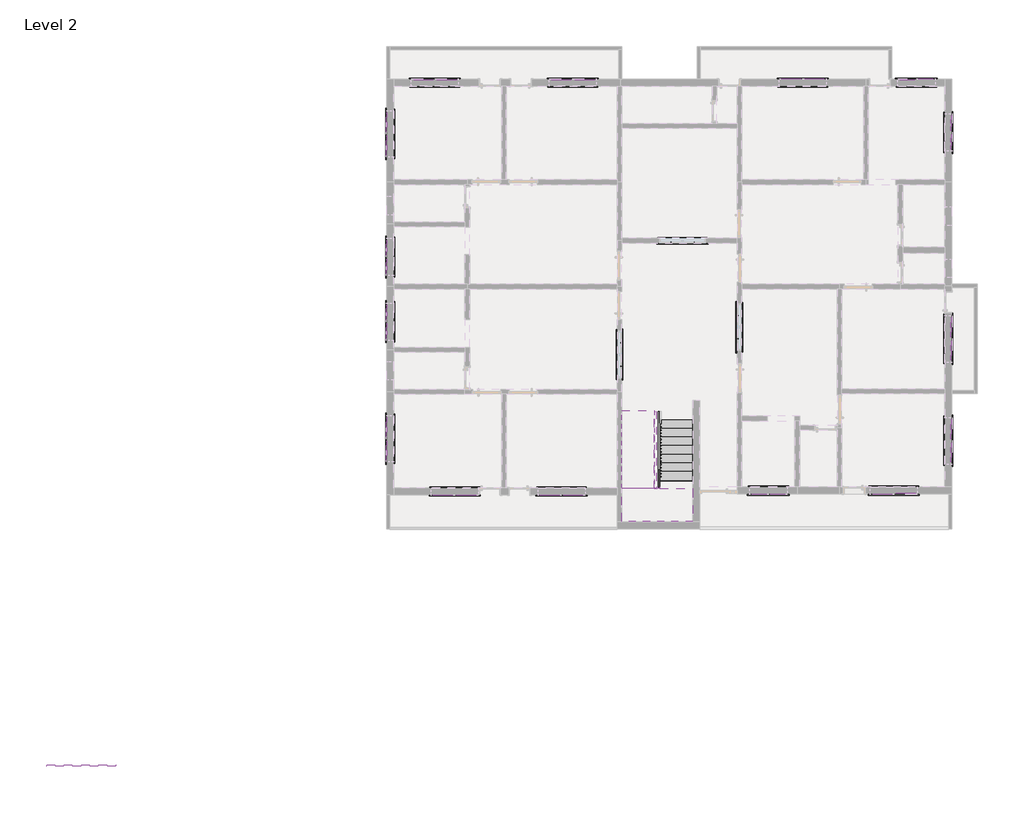
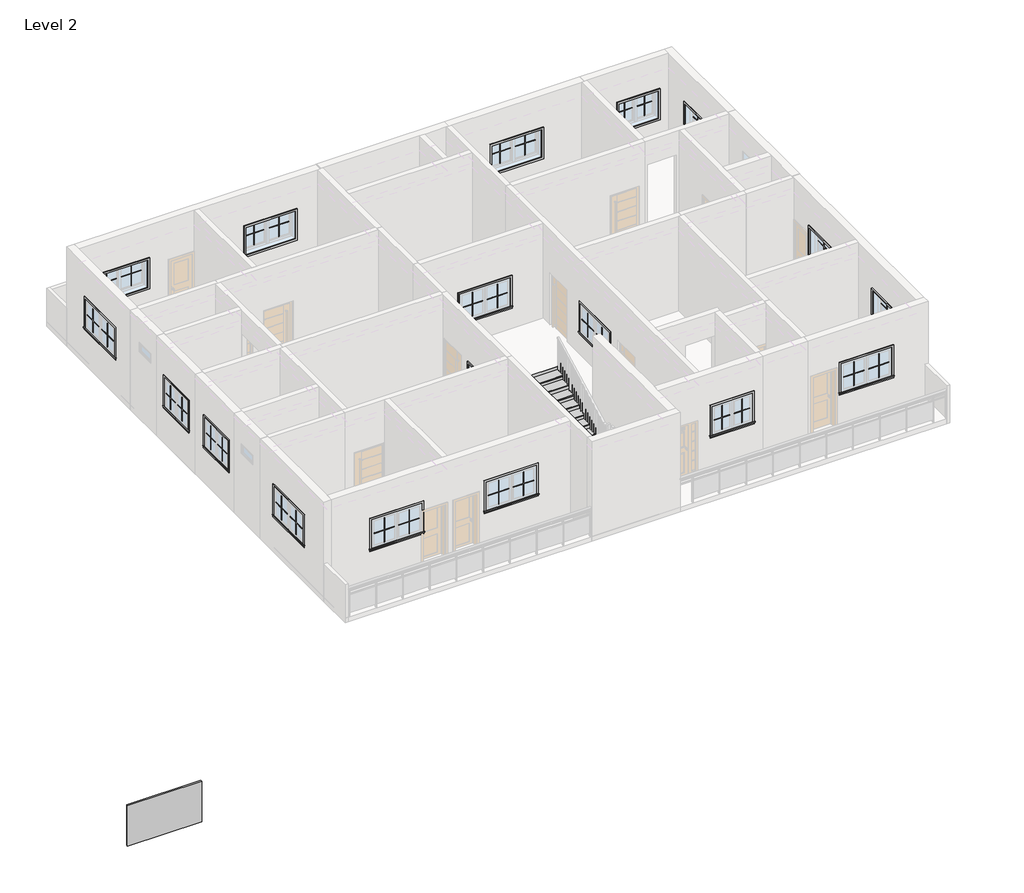
# One storey, part 5 of 5: 73 proxies, 3 members, 2 stair flights, 1 slab.
"""IFC4 building model written with IfcOpenShell, lengths in millimetres."""

from ifc_helpers import new_model, si_unit, frame, origin, place, context, project, spatial, polyline, outline, extrude, transform, mapped, element, save
from components import flag_flag_4961f895, m_muntin_pattern_2x2_m_muntin_pattern_2x2_9352d081, m_muntin_pattern_2x2_m_muntin_pattern_2x2_5c2cbe28, m_muntin_pattern_2x2_m_muntin_pattern_2x2_2357e71d, m_muntin_pattern_2x2_m_muntin_pattern_2x2_302d8f29, m_trim_window_exterior_flat_with_sill_e3533f3c, m_trim_window_exterior_flat_with_sill_6ae8fed8, m_trim_window_interior_flat_picture_frame_7d8195fd, m_trim_window_interior_flat_picture_frame_fffd0b6f, non_monolithic_landing_175d1c90, stair_flight_4edc9e4a, stair_flight_4fea8275

model = new_model("IFC4")

# Units and contexts
model_context = context("Model", 3, world=origin())
ifc_project = project(units=[si_unit("LENGTHUNIT", "METRE", prefix="MILLI")], contexts=[model_context])

# Site, building, storey
site = spatial("IfcSite", under=ifc_project)
building = spatial("IfcBuilding", under=site)
storey = spatial("IfcBuildingStorey", under=building, Name="Level 2", Elevation=3200.4)

# Proxies
placement = place(None, origin())
flag_flag_shape = flag_flag_4961f895(model_context)
element("IfcBuildingElementProxy", 1, Name="FLAG : FLAG", ObjectType="FLAG : FLAG", at=placement, inside=storey, context=model_context, shape_type="MappedRepresentation", body=[
    mapped(flag_flag_shape, transform((0.0, 0.0, 0.0), x_axis=(1.0, 0.0, 0.0), y_axis=(0.0, 1.0, 0.0), z_axis=(0.0, 0.0, 1.0))),
])
m_muntin_pattern_2x2_m_muntin_pattern_2x2_shape = m_muntin_pattern_2x2_m_muntin_pattern_2x2_9352d081(model_context)
element("IfcBuildingElementProxy", 2, Name="M_Muntin Pattern_2x2 : M_Muntin Pattern_2x2", ObjectType="M_Muntin Pattern_2x2 : M_Muntin Pattern_2x2", at=placement, inside=storey, context=model_context, shape_type="MappedRepresentation", body=[
    mapped(m_muntin_pattern_2x2_m_muntin_pattern_2x2_shape, transform((-23821.9972893, 23321.4672903, 4489.4070312), x_axis=(1.0, 0.0, 0.0), y_axis=(0.0, 1.0, 0.0), z_axis=(0.0, 0.0, 1.0))),
])
element("IfcBuildingElementProxy", 3, Name="M_Muntin Pattern_2x2 : M_Muntin Pattern_2x2", ObjectType="M_Muntin Pattern_2x2 : M_Muntin Pattern_2x2", at=placement, inside=storey, context=model_context, shape_type="MappedRepresentation", body=[
    mapped(m_muntin_pattern_2x2_m_muntin_pattern_2x2_shape, transform((-24995.1597893, 21173.5797903, 4489.4070312), x_axis=(0.0, 1.0, 0.0), y_axis=(-1.0, 0.0, 0.0), z_axis=(0.0, 0.0, 1.0))),
])
element("IfcBuildingElementProxy", 4, Name="M_Muntin Pattern_2x2 : M_Muntin Pattern_2x2", ObjectType="M_Muntin Pattern_2x2 : M_Muntin Pattern_2x2", at=placement, inside=storey, context=model_context, shape_type="MappedRepresentation", body=[
    mapped(m_muntin_pattern_2x2_m_muntin_pattern_2x2_shape, transform((-24995.1597893, 11242.1797903, 4489.4070312), x_axis=(0.0, 1.0, 0.0), y_axis=(-1.0, 0.0, 0.0), z_axis=(0.0, 0.0, 1.0))),
])
element("IfcBuildingElementProxy", 5, Name="M_Muntin Pattern_2x2 : M_Muntin Pattern_2x2", ObjectType="M_Muntin Pattern_2x2 : M_Muntin Pattern_2x2", at=placement, inside=storey, context=model_context, shape_type="MappedRepresentation", body=[
    mapped(m_muntin_pattern_2x2_m_muntin_pattern_2x2_shape, transform((-22415.4722893, 9802.3172903, 4489.4070312), x_axis=(-1.0, 0.0, 0.0), y_axis=(0.0, -1.0, 0.0), z_axis=(0.0, 0.0, 1.0))),
])
element("IfcBuildingElementProxy", 6, Name="M_Muntin Pattern_2x2 : M_Muntin Pattern_2x2", ObjectType="M_Muntin Pattern_2x2 : M_Muntin Pattern_2x2", at=placement, inside=storey, context=model_context, shape_type="MappedRepresentation", body=[
    mapped(m_muntin_pattern_2x2_m_muntin_pattern_2x2_shape, transform((-18935.6722893, 9802.3172903, 4489.4070312), x_axis=(-1.0, 0.0, 0.0), y_axis=(0.0, -1.0, 0.0), z_axis=(0.0, 0.0, 1.0))),
])
element("IfcBuildingElementProxy", 7, Name="M_Muntin Pattern_2x2 : M_Muntin Pattern_2x2", ObjectType="M_Muntin Pattern_2x2 : M_Muntin Pattern_2x2", at=placement, inside=storey, context=model_context, shape_type="MappedRepresentation", body=[
    mapped(m_muntin_pattern_2x2_m_muntin_pattern_2x2_shape, transform((-8121.6222893, 9827.7172903, 4489.4070312), x_axis=(-1.0, 0.0, 0.0), y_axis=(0.0, -1.0, 0.0), z_axis=(0.0, 0.0, 1.0))),
])
element("IfcBuildingElementProxy", 8, Name="M_Muntin Pattern_2x2 : M_Muntin Pattern_2x2", ObjectType="M_Muntin Pattern_2x2 : M_Muntin Pattern_2x2", at=placement, inside=storey, context=model_context, shape_type="MappedRepresentation", body=[
    mapped(m_muntin_pattern_2x2_m_muntin_pattern_2x2_shape, transform((-6624.6097893, 11931.1547903, 4489.4070312), x_axis=(0.0, -1.0, 0.0), y_axis=(1.0, 0.0, 0.0), z_axis=(0.0, 0.0, 1.0))),
])
element("IfcBuildingElementProxy", 9, Name="M_Muntin Pattern_2x2 : M_Muntin Pattern_2x2", ObjectType="M_Muntin Pattern_2x2 : M_Muntin Pattern_2x2", at=placement, inside=storey, context=model_context, shape_type="MappedRepresentation", body=[
    mapped(m_muntin_pattern_2x2_m_muntin_pattern_2x2_shape, transform((-6624.6097893, 15252.2047903, 4489.4070312), x_axis=(0.0, -1.0, 0.0), y_axis=(1.0, 0.0, 0.0), z_axis=(0.0, 0.0, 1.0))),
])
element("IfcBuildingElementProxy", 10, Name="M_Muntin Pattern_2x2 : M_Muntin Pattern_2x2", ObjectType="M_Muntin Pattern_2x2 : M_Muntin Pattern_2x2", at=placement, inside=storey, context=model_context, shape_type="MappedRepresentation", body=[
    mapped(m_muntin_pattern_2x2_m_muntin_pattern_2x2_shape, transform((-11845.8972893, 23321.4672903, 4489.4070312), x_axis=(1.0, 0.0, 0.0), y_axis=(0.0, 1.0, 0.0), z_axis=(0.0, 0.0, 1.0))),
])
element("IfcBuildingElementProxy", 11, Name="M_Muntin Pattern_2x2 : M_Muntin Pattern_2x2", ObjectType="M_Muntin Pattern_2x2 : M_Muntin Pattern_2x2", at=placement, inside=storey, context=model_context, shape_type="MappedRepresentation", body=[
    mapped(m_muntin_pattern_2x2_m_muntin_pattern_2x2_shape, transform((-19332.5472893, 23321.4672903, 4489.4070312), x_axis=(1.0, 0.0, 0.0), y_axis=(0.0, 1.0, 0.0), z_axis=(0.0, 0.0, 1.0))),
])
element("IfcBuildingElementProxy", 12, Name="M_Muntin Pattern_2x2 : M_Muntin Pattern_2x2", ObjectType="M_Muntin Pattern_2x2 : M_Muntin Pattern_2x2", at=placement, inside=storey, context=model_context, shape_type="MappedRepresentation", body=[
    mapped(m_muntin_pattern_2x2_m_muntin_pattern_2x2_shape, transform((-14998.6722893, 18006.5172903, 4170.25), x_axis=(-1.0, 0.0, 0.0), y_axis=(0.0, -1.0, 0.0), z_axis=(0.0, 0.0, 1.0))),
])
element("IfcBuildingElementProxy", 13, Name="M_Muntin Pattern_2x2 : M_Muntin Pattern_2x2", ObjectType="M_Muntin Pattern_2x2 : M_Muntin Pattern_2x2", at=placement, inside=storey, context=model_context, shape_type="MappedRepresentation", body=[
    mapped(m_muntin_pattern_2x2_m_muntin_pattern_2x2_shape, transform((-17368.8097893, 14744.2047903, 4170.25), x_axis=(0.0, -1.0, 0.0), y_axis=(1.0, 0.0, 0.0), z_axis=(0.0, 0.0, 1.0))),
])
element("IfcBuildingElementProxy", 14, Name="M_Muntin Pattern_2x2 : M_Muntin Pattern_2x2", ObjectType="M_Muntin Pattern_2x2 : M_Muntin Pattern_2x2", at=placement, inside=storey, context=model_context, shape_type="MappedRepresentation", body=[
    mapped(m_muntin_pattern_2x2_m_muntin_pattern_2x2_shape, transform((-13590.5597893, 14874.3797903, 4170.25), x_axis=(0.0, 1.0, 0.0), y_axis=(-1.0, 0.0, 0.0), z_axis=(0.0, 0.0, 1.0))),
])
m_muntin_pattern_2x2_m_muntin_pattern_2x2_2_shape = m_muntin_pattern_2x2_m_muntin_pattern_2x2_5c2cbe28(model_context)
element("IfcBuildingElementProxy", 15, Name="M_Muntin Pattern_2x2 : M_Muntin Pattern_2x2", ObjectType="M_Muntin Pattern_2x2 : M_Muntin Pattern_2x2", at=placement, inside=storey, context=model_context, shape_type="MappedRepresentation", body=[
    mapped(m_muntin_pattern_2x2_m_muntin_pattern_2x2_2_shape, transform((-23063.1722893, 23321.4672903, 4489.4070313), x_axis=(-1.0, 0.0, 0.0), y_axis=(0.0, -1.0, 0.0), z_axis=(0.0, 0.0, 1.0))),
])
element("IfcBuildingElementProxy", 16, Name="M_Muntin Pattern_2x2 : M_Muntin Pattern_2x2", ObjectType="M_Muntin Pattern_2x2 : M_Muntin Pattern_2x2", at=placement, inside=storey, context=model_context, shape_type="MappedRepresentation", body=[
    mapped(m_muntin_pattern_2x2_m_muntin_pattern_2x2_2_shape, transform((-24995.1597893, 21932.4047903, 4489.4070313), x_axis=(0.0, -1.0, 0.0), y_axis=(1.0, 0.0, 0.0), z_axis=(0.0, 0.0, 1.0))),
])
element("IfcBuildingElementProxy", 17, Name="M_Muntin Pattern_2x2 : M_Muntin Pattern_2x2", ObjectType="M_Muntin Pattern_2x2 : M_Muntin Pattern_2x2", at=placement, inside=storey, context=model_context, shape_type="MappedRepresentation", body=[
    mapped(m_muntin_pattern_2x2_m_muntin_pattern_2x2_2_shape, transform((-24995.1597893, 12001.0047903, 4489.4070313), x_axis=(0.0, -1.0, 0.0), y_axis=(1.0, 0.0, 0.0), z_axis=(0.0, 0.0, 1.0))),
])
element("IfcBuildingElementProxy", 18, Name="M_Muntin Pattern_2x2 : M_Muntin Pattern_2x2", ObjectType="M_Muntin Pattern_2x2 : M_Muntin Pattern_2x2", at=placement, inside=storey, context=model_context, shape_type="MappedRepresentation", body=[
    mapped(m_muntin_pattern_2x2_m_muntin_pattern_2x2_2_shape, transform((-23174.2972893, 9802.3172903, 4489.4070313), x_axis=(1.0, 0.0, 0.0), y_axis=(0.0, 1.0, 0.0), z_axis=(0.0, 0.0, 1.0))),
])
element("IfcBuildingElementProxy", 19, Name="M_Muntin Pattern_2x2 : M_Muntin Pattern_2x2", ObjectType="M_Muntin Pattern_2x2 : M_Muntin Pattern_2x2", at=placement, inside=storey, context=model_context, shape_type="MappedRepresentation", body=[
    mapped(m_muntin_pattern_2x2_m_muntin_pattern_2x2_2_shape, transform((-19694.4972893, 9802.3172903, 4489.4070313), x_axis=(1.0, 0.0, 0.0), y_axis=(0.0, 1.0, 0.0), z_axis=(0.0, 0.0, 1.0))),
])
element("IfcBuildingElementProxy", 20, Name="M_Muntin Pattern_2x2 : M_Muntin Pattern_2x2", ObjectType="M_Muntin Pattern_2x2 : M_Muntin Pattern_2x2", at=placement, inside=storey, context=model_context, shape_type="MappedRepresentation", body=[
    mapped(m_muntin_pattern_2x2_m_muntin_pattern_2x2_2_shape, transform((-8880.4472893, 9827.7172903, 4489.4070313), x_axis=(1.0, 0.0, 0.0), y_axis=(0.0, 1.0, 0.0), z_axis=(0.0, 0.0, 1.0))),
])
element("IfcBuildingElementProxy", 21, Name="M_Muntin Pattern_2x2 : M_Muntin Pattern_2x2", ObjectType="M_Muntin Pattern_2x2 : M_Muntin Pattern_2x2", at=placement, inside=storey, context=model_context, shape_type="MappedRepresentation", body=[
    mapped(m_muntin_pattern_2x2_m_muntin_pattern_2x2_2_shape, transform((-6624.6097893, 11172.3297903, 4489.4070313), x_axis=(0.0, 1.0, 0.0), y_axis=(-1.0, 0.0, 0.0), z_axis=(0.0, 0.0, 1.0))),
])
element("IfcBuildingElementProxy", 22, Name="M_Muntin Pattern_2x2 : M_Muntin Pattern_2x2", ObjectType="M_Muntin Pattern_2x2 : M_Muntin Pattern_2x2", at=placement, inside=storey, context=model_context, shape_type="MappedRepresentation", body=[
    mapped(m_muntin_pattern_2x2_m_muntin_pattern_2x2_2_shape, transform((-6624.6097893, 14493.3797903, 4489.4070313), x_axis=(0.0, 1.0, 0.0), y_axis=(-1.0, 0.0, 0.0), z_axis=(0.0, 0.0, 1.0))),
])
element("IfcBuildingElementProxy", 23, Name="M_Muntin Pattern_2x2 : M_Muntin Pattern_2x2", ObjectType="M_Muntin Pattern_2x2 : M_Muntin Pattern_2x2", at=placement, inside=storey, context=model_context, shape_type="MappedRepresentation", body=[
    mapped(m_muntin_pattern_2x2_m_muntin_pattern_2x2_2_shape, transform((-11087.0722893, 23321.4672903, 4489.4070313), x_axis=(-1.0, 0.0, 0.0), y_axis=(0.0, -1.0, 0.0), z_axis=(0.0, 0.0, 1.0))),
])
element("IfcBuildingElementProxy", 24, Name="M_Muntin Pattern_2x2 : M_Muntin Pattern_2x2", ObjectType="M_Muntin Pattern_2x2 : M_Muntin Pattern_2x2", at=placement, inside=storey, context=model_context, shape_type="MappedRepresentation", body=[
    mapped(m_muntin_pattern_2x2_m_muntin_pattern_2x2_2_shape, transform((-18573.7222893, 23321.4672903, 4489.4070313), x_axis=(-1.0, 0.0, 0.0), y_axis=(0.0, -1.0, 0.0), z_axis=(0.0, 0.0, 1.0))),
])
element("IfcBuildingElementProxy", 25, Name="M_Muntin Pattern_2x2 : M_Muntin Pattern_2x2", ObjectType="M_Muntin Pattern_2x2 : M_Muntin Pattern_2x2", at=placement, inside=storey, context=model_context, shape_type="MappedRepresentation", body=[
    mapped(m_muntin_pattern_2x2_m_muntin_pattern_2x2_2_shape, transform((-15757.4972893, 18006.5172903, 4170.25), x_axis=(1.0, 0.0, 0.0), y_axis=(0.0, 1.0, 0.0), z_axis=(0.0, 0.0, 1.0))),
])
element("IfcBuildingElementProxy", 26, Name="M_Muntin Pattern_2x2 : M_Muntin Pattern_2x2", ObjectType="M_Muntin Pattern_2x2 : M_Muntin Pattern_2x2", at=placement, inside=storey, context=model_context, shape_type="MappedRepresentation", body=[
    mapped(m_muntin_pattern_2x2_m_muntin_pattern_2x2_2_shape, transform((-17368.8097893, 13985.3797903, 4170.25), x_axis=(0.0, 1.0, 0.0), y_axis=(-1.0, 0.0, 0.0), z_axis=(0.0, 0.0, 1.0))),
])
element("IfcBuildingElementProxy", 27, Name="M_Muntin Pattern_2x2 : M_Muntin Pattern_2x2", ObjectType="M_Muntin Pattern_2x2 : M_Muntin Pattern_2x2", at=placement, inside=storey, context=model_context, shape_type="MappedRepresentation", body=[
    mapped(m_muntin_pattern_2x2_m_muntin_pattern_2x2_2_shape, transform((-13590.5597893, 15633.2047903, 4170.25), x_axis=(0.0, -1.0, 0.0), y_axis=(1.0, 0.0, 0.0), z_axis=(0.0, 0.0, 1.0))),
])
m_muntin_pattern_2x2_m_muntin_pattern_2x2_3_shape = m_muntin_pattern_2x2_m_muntin_pattern_2x2_2357e71d(model_context)
element("IfcBuildingElementProxy", 28, Name="M_Muntin Pattern_2x2 : M_Muntin Pattern_2x2", ObjectType="M_Muntin Pattern_2x2 : M_Muntin Pattern_2x2", at=placement, inside=storey, context=model_context, shape_type="MappedRepresentation", body=[
    mapped(m_muntin_pattern_2x2_m_muntin_pattern_2x2_3_shape, transform((-24995.1597893, 17236.5797903, 4489.45), x_axis=(0.0, 1.0, 0.0), y_axis=(-1.0, 0.0, 0.0), z_axis=(0.0, 0.0, 1.0))),
])
element("IfcBuildingElementProxy", 29, Name="M_Muntin Pattern_2x2 : M_Muntin Pattern_2x2", ObjectType="M_Muntin Pattern_2x2 : M_Muntin Pattern_2x2", at=placement, inside=storey, context=model_context, shape_type="MappedRepresentation", body=[
    mapped(m_muntin_pattern_2x2_m_muntin_pattern_2x2_3_shape, transform((-24995.1597893, 15128.3797903, 4489.45), x_axis=(0.0, 1.0, 0.0), y_axis=(-1.0, 0.0, 0.0), z_axis=(0.0, 0.0, 1.0))),
])
element("IfcBuildingElementProxy", 30, Name="M_Muntin Pattern_2x2 : M_Muntin Pattern_2x2", ObjectType="M_Muntin Pattern_2x2 : M_Muntin Pattern_2x2", at=placement, inside=storey, context=model_context, shape_type="MappedRepresentation", body=[
    mapped(m_muntin_pattern_2x2_m_muntin_pattern_2x2_3_shape, transform((-12280.8722893, 9827.7172903, 4489.45), x_axis=(-1.0, 0.0, 0.0), y_axis=(0.0, -1.0, 0.0), z_axis=(0.0, 0.0, 1.0))),
])
element("IfcBuildingElementProxy", 31, Name="M_Muntin Pattern_2x2 : M_Muntin Pattern_2x2", ObjectType="M_Muntin Pattern_2x2 : M_Muntin Pattern_2x2", at=placement, inside=storey, context=model_context, shape_type="MappedRepresentation", body=[
    mapped(m_muntin_pattern_2x2_m_muntin_pattern_2x2_3_shape, transform((-6624.6097893, 21900.6547903, 4489.45), x_axis=(0.0, -1.0, 0.0), y_axis=(1.0, 0.0, 0.0), z_axis=(0.0, 0.0, 1.0))),
])
element("IfcBuildingElementProxy", 32, Name="M_Muntin Pattern_2x2 : M_Muntin Pattern_2x2", ObjectType="M_Muntin Pattern_2x2 : M_Muntin Pattern_2x2", at=placement, inside=storey, context=model_context, shape_type="MappedRepresentation", body=[
    mapped(m_muntin_pattern_2x2_m_muntin_pattern_2x2_3_shape, transform((-8067.6472893, 23321.4672903, 4489.45), x_axis=(1.0, 0.0, 0.0), y_axis=(0.0, 1.0, 0.0), z_axis=(0.0, 0.0, 1.0))),
])
m_muntin_pattern_2x2_m_muntin_pattern_2x2_4_shape = m_muntin_pattern_2x2_m_muntin_pattern_2x2_302d8f29(model_context)
element("IfcBuildingElementProxy", 33, Name="M_Muntin Pattern_2x2 : M_Muntin Pattern_2x2", ObjectType="M_Muntin Pattern_2x2 : M_Muntin Pattern_2x2", at=placement, inside=storey, context=model_context, shape_type="MappedRepresentation", body=[
    mapped(m_muntin_pattern_2x2_m_muntin_pattern_2x2_4_shape, transform((-24995.1597893, 17843.0047903, 4489.45), x_axis=(0.0, -1.0, 0.0), y_axis=(1.0, 0.0, 0.0), z_axis=(0.0, 0.0, 1.0))),
])
element("IfcBuildingElementProxy", 34, Name="M_Muntin Pattern_2x2 : M_Muntin Pattern_2x2", ObjectType="M_Muntin Pattern_2x2 : M_Muntin Pattern_2x2", at=placement, inside=storey, context=model_context, shape_type="MappedRepresentation", body=[
    mapped(m_muntin_pattern_2x2_m_muntin_pattern_2x2_4_shape, transform((-24995.1597893, 15734.8047903, 4489.45), x_axis=(0.0, -1.0, 0.0), y_axis=(1.0, 0.0, 0.0), z_axis=(0.0, 0.0, 1.0))),
])
element("IfcBuildingElementProxy", 35, Name="M_Muntin Pattern_2x2 : M_Muntin Pattern_2x2", ObjectType="M_Muntin Pattern_2x2 : M_Muntin Pattern_2x2", at=placement, inside=storey, context=model_context, shape_type="MappedRepresentation", body=[
    mapped(m_muntin_pattern_2x2_m_muntin_pattern_2x2_4_shape, transform((-12887.2972893, 9827.7172903, 4489.45), x_axis=(1.0, 0.0, 0.0), y_axis=(0.0, 1.0, 0.0), z_axis=(0.0, 0.0, 1.0))),
])
element("IfcBuildingElementProxy", 36, Name="M_Muntin Pattern_2x2 : M_Muntin Pattern_2x2", ObjectType="M_Muntin Pattern_2x2 : M_Muntin Pattern_2x2", at=placement, inside=storey, context=model_context, shape_type="MappedRepresentation", body=[
    mapped(m_muntin_pattern_2x2_m_muntin_pattern_2x2_4_shape, transform((-6624.6097893, 21294.2297903, 4489.45), x_axis=(0.0, 1.0, 0.0), y_axis=(-1.0, 0.0, 0.0), z_axis=(0.0, 0.0, 1.0))),
])
element("IfcBuildingElementProxy", 37, Name="M_Muntin Pattern_2x2 : M_Muntin Pattern_2x2", ObjectType="M_Muntin Pattern_2x2 : M_Muntin Pattern_2x2", at=placement, inside=storey, context=model_context, shape_type="MappedRepresentation", body=[
    mapped(m_muntin_pattern_2x2_m_muntin_pattern_2x2_4_shape, transform((-7461.2222893, 23321.4672903, 4489.45), x_axis=(-1.0, 0.0, 0.0), y_axis=(0.0, -1.0, 0.0), z_axis=(0.0, 0.0, 1.0))),
])
m_trim_window_exterior_flat_with_sill_shape = m_trim_window_exterior_flat_with_sill_e3533f3c(model_context)
element("IfcBuildingElementProxy", 38, Name="M_Trim-Window-Exterior-Flat : with Sill", ObjectType="M_Trim-Window-Exterior-Flat : with Sill", at=placement, inside=storey, context=model_context, shape_type="MappedRepresentation", body=[
    mapped(m_trim_window_exterior_flat_with_sill_shape, transform((-23442.5847893, 23330.9922903, 5333.9570313), x_axis=(-1.0, 0.0, 0.0), y_axis=(0.0, 0.0, 1.0), z_axis=(0.0, 1.0, 0.0))),
])
element("IfcBuildingElementProxy", 39, Name="M_Trim-Window-Exterior-Flat : with Sill", ObjectType="M_Trim-Window-Exterior-Flat : with Sill", at=placement, inside=storey, context=model_context, shape_type="MappedRepresentation", body=[
    mapped(m_trim_window_exterior_flat_with_sill_shape, transform((-25004.6847893, 21552.9922903, 5333.9570313), x_axis=(0.0, -1.0, 0.0), y_axis=(0.0, 0.0, 1.0), z_axis=(-1.0, 0.0, 0.0))),
])
element("IfcBuildingElementProxy", 40, Name="M_Trim-Window-Exterior-Flat : with Sill", ObjectType="M_Trim-Window-Exterior-Flat : with Sill", at=placement, inside=storey, context=model_context, shape_type="MappedRepresentation", body=[
    mapped(m_trim_window_exterior_flat_with_sill_shape, transform((-25004.6847893, 11621.5922903, 5333.9570313), x_axis=(0.0, -1.0, 0.0), y_axis=(0.0, 0.0, 1.0), z_axis=(-1.0, 0.0, 0.0))),
])
element("IfcBuildingElementProxy", 41, Name="M_Trim-Window-Exterior-Flat : with Sill", ObjectType="M_Trim-Window-Exterior-Flat : with Sill", at=placement, inside=storey, context=model_context, shape_type="MappedRepresentation", body=[
    mapped(m_trim_window_exterior_flat_with_sill_shape, transform((-22794.8847893, 9792.7922903, 5333.9570313), x_axis=(1.0, 0.0, 0.0), y_axis=(0.0, 0.0, 1.0), z_axis=(0.0, -1.0, 0.0))),
])
element("IfcBuildingElementProxy", 42, Name="M_Trim-Window-Exterior-Flat : with Sill", ObjectType="M_Trim-Window-Exterior-Flat : with Sill", at=placement, inside=storey, context=model_context, shape_type="MappedRepresentation", body=[
    mapped(m_trim_window_exterior_flat_with_sill_shape, transform((-19315.0847893, 9792.7922903, 5333.9570313), x_axis=(1.0, 0.0, 0.0), y_axis=(0.0, 0.0, 1.0), z_axis=(0.0, -1.0, 0.0))),
])
element("IfcBuildingElementProxy", 43, Name="M_Trim-Window-Exterior-Flat : with Sill", ObjectType="M_Trim-Window-Exterior-Flat : with Sill", at=placement, inside=storey, context=model_context, shape_type="MappedRepresentation", body=[
    mapped(m_trim_window_exterior_flat_with_sill_shape, transform((-8501.0347893, 9818.1922903, 5333.9570313), x_axis=(1.0, 0.0, 0.0), y_axis=(0.0, 0.0, 1.0), z_axis=(0.0, -1.0, 0.0))),
])
element("IfcBuildingElementProxy", 44, Name="M_Trim-Window-Exterior-Flat : with Sill", ObjectType="M_Trim-Window-Exterior-Flat : with Sill", at=placement, inside=storey, context=model_context, shape_type="MappedRepresentation", body=[
    mapped(m_trim_window_exterior_flat_with_sill_shape, transform((-6615.0847893, 11551.7422903, 5333.9570313), x_axis=(0.0, 1.0, 0.0), y_axis=(0.0, 0.0, 1.0), z_axis=(1.0, 0.0, 0.0))),
])
element("IfcBuildingElementProxy", 45, Name="M_Trim-Window-Exterior-Flat : with Sill", ObjectType="M_Trim-Window-Exterior-Flat : with Sill", at=placement, inside=storey, context=model_context, shape_type="MappedRepresentation", body=[
    mapped(m_trim_window_exterior_flat_with_sill_shape, transform((-6615.0847893, 14872.7922903, 5333.9570313), x_axis=(0.0, 1.0, 0.0), y_axis=(0.0, 0.0, 1.0), z_axis=(1.0, 0.0, 0.0))),
])
element("IfcBuildingElementProxy", 46, Name="M_Trim-Window-Exterior-Flat : with Sill", ObjectType="M_Trim-Window-Exterior-Flat : with Sill", at=placement, inside=storey, context=model_context, shape_type="MappedRepresentation", body=[
    mapped(m_trim_window_exterior_flat_with_sill_shape, transform((-11466.4847893, 23330.9922903, 5333.9570313), x_axis=(-1.0, 0.0, 0.0), y_axis=(0.0, 0.0, 1.0), z_axis=(0.0, 1.0, 0.0))),
])
element("IfcBuildingElementProxy", 47, Name="M_Trim-Window-Exterior-Flat : with Sill", ObjectType="M_Trim-Window-Exterior-Flat : with Sill", at=placement, inside=storey, context=model_context, shape_type="MappedRepresentation", body=[
    mapped(m_trim_window_exterior_flat_with_sill_shape, transform((-18953.1347893, 23330.9922903, 5333.9570313), x_axis=(-1.0, 0.0, 0.0), y_axis=(0.0, 0.0, 1.0), z_axis=(0.0, 1.0, 0.0))),
])
element("IfcBuildingElementProxy", 48, Name="M_Trim-Window-Exterior-Flat : with Sill", ObjectType="M_Trim-Window-Exterior-Flat : with Sill", at=placement, inside=storey, context=model_context, shape_type="MappedRepresentation", body=[
    mapped(m_trim_window_exterior_flat_with_sill_shape, transform((-15378.0847893, 17996.9922903, 5014.8), x_axis=(1.0, 0.0, 0.0), y_axis=(0.0, 0.0, 1.0), z_axis=(0.0, -1.0, 0.0))),
])
element("IfcBuildingElementProxy", 49, Name="M_Trim-Window-Exterior-Flat : with Sill", ObjectType="M_Trim-Window-Exterior-Flat : with Sill", at=placement, inside=storey, context=model_context, shape_type="MappedRepresentation", body=[
    mapped(m_trim_window_exterior_flat_with_sill_shape, transform((-17359.2847893, 14364.7922903, 5014.8), x_axis=(0.0, 1.0, 0.0), y_axis=(0.0, 0.0, 1.0), z_axis=(1.0, 0.0, 0.0))),
])
element("IfcBuildingElementProxy", 50, Name="M_Trim-Window-Exterior-Flat : with Sill", ObjectType="M_Trim-Window-Exterior-Flat : with Sill", at=placement, inside=storey, context=model_context, shape_type="MappedRepresentation", body=[
    mapped(m_trim_window_exterior_flat_with_sill_shape, transform((-13600.0847893, 15253.7922903, 5014.8), x_axis=(0.0, -1.0, 0.0), y_axis=(0.0, 0.0, 1.0), z_axis=(-1.0, 0.0, 0.0))),
])
m_trim_window_exterior_flat_with_sill_2_shape = m_trim_window_exterior_flat_with_sill_6ae8fed8(model_context)
element("IfcBuildingElementProxy", 51, Name="M_Trim-Window-Exterior-Flat : with Sill", ObjectType="M_Trim-Window-Exterior-Flat : with Sill", at=placement, inside=storey, context=model_context, shape_type="MappedRepresentation", body=[
    mapped(m_trim_window_exterior_flat_with_sill_2_shape, transform((-25004.6847893, 17539.7922903, 5334.0), x_axis=(0.0, -1.0, 0.0), y_axis=(0.0, 0.0, 1.0), z_axis=(-1.0, 0.0, 0.0))),
])
element("IfcBuildingElementProxy", 52, Name="M_Trim-Window-Exterior-Flat : with Sill", ObjectType="M_Trim-Window-Exterior-Flat : with Sill", at=placement, inside=storey, context=model_context, shape_type="MappedRepresentation", body=[
    mapped(m_trim_window_exterior_flat_with_sill_2_shape, transform((-25004.6847893, 15431.5922903, 5334.0), x_axis=(0.0, -1.0, 0.0), y_axis=(0.0, 0.0, 1.0), z_axis=(-1.0, 0.0, 0.0))),
])
element("IfcBuildingElementProxy", 53, Name="M_Trim-Window-Exterior-Flat : with Sill", ObjectType="M_Trim-Window-Exterior-Flat : with Sill", at=placement, inside=storey, context=model_context, shape_type="MappedRepresentation", body=[
    mapped(m_trim_window_exterior_flat_with_sill_2_shape, transform((-12584.0847893, 9818.1922903, 5334.0), x_axis=(1.0, 0.0, 0.0), y_axis=(0.0, 0.0, 1.0), z_axis=(0.0, -1.0, 0.0))),
])
element("IfcBuildingElementProxy", 54, Name="M_Trim-Window-Exterior-Flat : with Sill", ObjectType="M_Trim-Window-Exterior-Flat : with Sill", at=placement, inside=storey, context=model_context, shape_type="MappedRepresentation", body=[
    mapped(m_trim_window_exterior_flat_with_sill_2_shape, transform((-6615.0847893, 21597.4422903, 5334.0), x_axis=(0.0, 1.0, 0.0), y_axis=(0.0, 0.0, 1.0), z_axis=(1.0, 0.0, 0.0))),
])
element("IfcBuildingElementProxy", 55, Name="M_Trim-Window-Exterior-Flat : with Sill", ObjectType="M_Trim-Window-Exterior-Flat : with Sill", at=placement, inside=storey, context=model_context, shape_type="MappedRepresentation", body=[
    mapped(m_trim_window_exterior_flat_with_sill_2_shape, transform((-7764.4347893, 23330.9922903, 5334.0), x_axis=(-1.0, 0.0, 0.0), y_axis=(0.0, 0.0, 1.0), z_axis=(0.0, 1.0, 0.0))),
])
m_trim_window_interior_flat_picture_frame_shape = m_trim_window_interior_flat_picture_frame_7d8195fd(model_context)
element("IfcBuildingElementProxy", 56, Name="M_Trim-Window-Interior-Flat : Picture Frame", ObjectType="M_Trim-Window-Interior-Flat : Picture Frame", at=placement, inside=storey, context=model_context, shape_type="MappedRepresentation", body=[
    mapped(m_trim_window_interior_flat_picture_frame_shape, transform((-23442.5847893, 23102.3922903, 5333.9570313), x_axis=(1.0, 0.0, 0.0), y_axis=(0.0, 0.0, 1.0), z_axis=(0.0, -1.0, 0.0))),
])
element("IfcBuildingElementProxy", 57, Name="M_Trim-Window-Interior-Flat : Picture Frame", ObjectType="M_Trim-Window-Interior-Flat : Picture Frame", at=placement, inside=storey, context=model_context, shape_type="MappedRepresentation", body=[
    mapped(m_trim_window_interior_flat_picture_frame_shape, transform((-24776.0847893, 21552.9922903, 5333.9570313), x_axis=(0.0, 1.0, 0.0), y_axis=(0.0, 0.0, 1.0), z_axis=(1.0, 0.0, 0.0))),
])
element("IfcBuildingElementProxy", 58, Name="M_Trim-Window-Interior-Flat : Picture Frame", ObjectType="M_Trim-Window-Interior-Flat : Picture Frame", at=placement, inside=storey, context=model_context, shape_type="MappedRepresentation", body=[
    mapped(m_trim_window_interior_flat_picture_frame_shape, transform((-24776.0847893, 11621.5922903, 5333.9570313), x_axis=(0.0, 1.0, 0.0), y_axis=(0.0, 0.0, 1.0), z_axis=(1.0, 0.0, 0.0))),
])
element("IfcBuildingElementProxy", 59, Name="M_Trim-Window-Interior-Flat : Picture Frame", ObjectType="M_Trim-Window-Interior-Flat : Picture Frame", at=placement, inside=storey, context=model_context, shape_type="MappedRepresentation", body=[
    mapped(m_trim_window_interior_flat_picture_frame_shape, transform((-22794.8847893, 10021.3922903, 5333.9570313), x_axis=(-1.0, 0.0, 0.0), y_axis=(0.0, 0.0, 1.0), z_axis=(0.0, 1.0, 0.0))),
])
element("IfcBuildingElementProxy", 60, Name="M_Trim-Window-Interior-Flat : Picture Frame", ObjectType="M_Trim-Window-Interior-Flat : Picture Frame", at=placement, inside=storey, context=model_context, shape_type="MappedRepresentation", body=[
    mapped(m_trim_window_interior_flat_picture_frame_shape, transform((-19315.0847893, 10021.3922903, 5333.9570313), x_axis=(-1.0, 0.0, 0.0), y_axis=(0.0, 0.0, 1.0), z_axis=(0.0, 1.0, 0.0))),
])
element("IfcBuildingElementProxy", 61, Name="M_Trim-Window-Interior-Flat : Picture Frame", ObjectType="M_Trim-Window-Interior-Flat : Picture Frame", at=placement, inside=storey, context=model_context, shape_type="MappedRepresentation", body=[
    mapped(m_trim_window_interior_flat_picture_frame_shape, transform((-8501.0347893, 10046.7922903, 5333.9570313), x_axis=(-1.0, 0.0, 0.0), y_axis=(0.0, 0.0, 1.0), z_axis=(0.0, 1.0, 0.0))),
])
element("IfcBuildingElementProxy", 62, Name="M_Trim-Window-Interior-Flat : Picture Frame", ObjectType="M_Trim-Window-Interior-Flat : Picture Frame", at=placement, inside=storey, context=model_context, shape_type="MappedRepresentation", body=[
    mapped(m_trim_window_interior_flat_picture_frame_shape, transform((-6843.6847893, 11551.7422903, 5333.9570313), x_axis=(0.0, -1.0, 0.0), y_axis=(0.0, 0.0, 1.0), z_axis=(-1.0, 0.0, 0.0))),
])
element("IfcBuildingElementProxy", 63, Name="M_Trim-Window-Interior-Flat : Picture Frame", ObjectType="M_Trim-Window-Interior-Flat : Picture Frame", at=placement, inside=storey, context=model_context, shape_type="MappedRepresentation", body=[
    mapped(m_trim_window_interior_flat_picture_frame_shape, transform((-6843.6847893, 14872.7922903, 5333.9570313), x_axis=(0.0, -1.0, 0.0), y_axis=(0.0, 0.0, 1.0), z_axis=(-1.0, 0.0, 0.0))),
])
element("IfcBuildingElementProxy", 64, Name="M_Trim-Window-Interior-Flat : Picture Frame", ObjectType="M_Trim-Window-Interior-Flat : Picture Frame", at=placement, inside=storey, context=model_context, shape_type="MappedRepresentation", body=[
    mapped(m_trim_window_interior_flat_picture_frame_shape, transform((-11466.4847893, 23102.3922903, 5333.9570313), x_axis=(1.0, 0.0, 0.0), y_axis=(0.0, 0.0, 1.0), z_axis=(0.0, -1.0, 0.0))),
])
element("IfcBuildingElementProxy", 65, Name="M_Trim-Window-Interior-Flat : Picture Frame", ObjectType="M_Trim-Window-Interior-Flat : Picture Frame", at=placement, inside=storey, context=model_context, shape_type="MappedRepresentation", body=[
    mapped(m_trim_window_interior_flat_picture_frame_shape, transform((-18953.1347893, 23102.3922903, 5333.9570313), x_axis=(1.0, 0.0, 0.0), y_axis=(0.0, 0.0, 1.0), z_axis=(0.0, -1.0, 0.0))),
])
element("IfcBuildingElementProxy", 66, Name="M_Trim-Window-Interior-Flat : Picture Frame", ObjectType="M_Trim-Window-Interior-Flat : Picture Frame", at=placement, inside=storey, context=model_context, shape_type="MappedRepresentation", body=[
    mapped(m_trim_window_interior_flat_picture_frame_shape, transform((-15378.0847893, 18149.3922903, 5014.8), x_axis=(-1.0, 0.0, 0.0), y_axis=(0.0, 0.0, 1.0), z_axis=(0.0, 1.0, 0.0))),
])
element("IfcBuildingElementProxy", 67, Name="M_Trim-Window-Interior-Flat : Picture Frame", ObjectType="M_Trim-Window-Interior-Flat : Picture Frame", at=placement, inside=storey, context=model_context, shape_type="MappedRepresentation", body=[
    mapped(m_trim_window_interior_flat_picture_frame_shape, transform((-17511.6847893, 14364.7922903, 5014.8), x_axis=(0.0, -1.0, 0.0), y_axis=(0.0, 0.0, 1.0), z_axis=(-1.0, 0.0, 0.0))),
])
element("IfcBuildingElementProxy", 68, Name="M_Trim-Window-Interior-Flat : Picture Frame", ObjectType="M_Trim-Window-Interior-Flat : Picture Frame", at=placement, inside=storey, context=model_context, shape_type="MappedRepresentation", body=[
    mapped(m_trim_window_interior_flat_picture_frame_shape, transform((-13447.6847893, 15253.7922903, 5014.8), x_axis=(0.0, 1.0, 0.0), y_axis=(0.0, 0.0, 1.0), z_axis=(1.0, 0.0, 0.0))),
])
m_trim_window_interior_flat_picture_frame_2_shape = m_trim_window_interior_flat_picture_frame_fffd0b6f(model_context)
element("IfcBuildingElementProxy", 69, Name="M_Trim-Window-Interior-Flat : Picture Frame", ObjectType="M_Trim-Window-Interior-Flat : Picture Frame", at=placement, inside=storey, context=model_context, shape_type="MappedRepresentation", body=[
    mapped(m_trim_window_interior_flat_picture_frame_2_shape, transform((-24776.0847893, 17539.7922903, 5334.0), x_axis=(0.0, 1.0, 0.0), y_axis=(0.0, 0.0, 1.0), z_axis=(1.0, 0.0, 0.0))),
])
element("IfcBuildingElementProxy", 70, Name="M_Trim-Window-Interior-Flat : Picture Frame", ObjectType="M_Trim-Window-Interior-Flat : Picture Frame", at=placement, inside=storey, context=model_context, shape_type="MappedRepresentation", body=[
    mapped(m_trim_window_interior_flat_picture_frame_2_shape, transform((-24776.0847893, 15431.5922903, 5334.0), x_axis=(0.0, 1.0, 0.0), y_axis=(0.0, 0.0, 1.0), z_axis=(1.0, 0.0, 0.0))),
])
element("IfcBuildingElementProxy", 71, Name="M_Trim-Window-Interior-Flat : Picture Frame", ObjectType="M_Trim-Window-Interior-Flat : Picture Frame", at=placement, inside=storey, context=model_context, shape_type="MappedRepresentation", body=[
    mapped(m_trim_window_interior_flat_picture_frame_2_shape, transform((-12584.0847893, 10046.7922903, 5334.0), x_axis=(-1.0, 0.0, 0.0), y_axis=(0.0, 0.0, 1.0), z_axis=(0.0, 1.0, 0.0))),
])
element("IfcBuildingElementProxy", 72, Name="M_Trim-Window-Interior-Flat : Picture Frame", ObjectType="M_Trim-Window-Interior-Flat : Picture Frame", at=placement, inside=storey, context=model_context, shape_type="MappedRepresentation", body=[
    mapped(m_trim_window_interior_flat_picture_frame_2_shape, transform((-6843.6847893, 21597.4422903, 5334.0), x_axis=(0.0, -1.0, 0.0), y_axis=(0.0, 0.0, 1.0), z_axis=(-1.0, 0.0, 0.0))),
])
element("IfcBuildingElementProxy", 73, Name="M_Trim-Window-Interior-Flat : Picture Frame", ObjectType="M_Trim-Window-Interior-Flat : Picture Frame", at=placement, inside=storey, context=model_context, shape_type="MappedRepresentation", body=[
    mapped(m_trim_window_interior_flat_picture_frame_2_shape, transform((-7764.4347893, 23102.3922903, 5334.0), x_axis=(1.0, 0.0, 0.0), y_axis=(0.0, 0.0, 1.0), z_axis=(0.0, -1.0, 0.0))),
])

# Members
element("IfcMember", 74, ObjectType="Stringer - 2\" Width", at=placement, inside=storey, context=model_context, shape_type="SweptSolid", body=[
    extrude(outline(polyline([(12510.5922903, 3405.1167581), (12510.5922903, 3200.4), (12243.7728762, 3200.4), (10046.7922903, 4344.2824538), (10046.7922903, 4687.9217168), (12510.5922903, 3405.1167581)])), frame((-16165.4847893, 0.0, 0.0), z_axis=(1.0, 0.0, 0.0), x_axis=(0.0, 1.0, 0.0)), (0.0, 0.0, 1.0), 50.8),
])
element("IfcMember", 75, ObjectType="Stringer - 2\" Width", at=placement, inside=storey, context=model_context, shape_type="SweptSolid", body=[
    extrude(outline(polyline([(9995.9922903, 4516.2047679), (9995.9922903, 4859.8440309), (12510.5922903, 6169.0985763), (12510.5922903, 5825.4593133), (9995.9922903, 4516.2047679)])), frame((-16292.4847893, 0.0, 0.0), z_axis=(1.0, 0.0, 0.0), x_axis=(0.0, 1.0, 0.0)), (0.0, 0.0, 1.0), 50.8),
])
element("IfcMember", 76, ObjectType="Stringer - 2\" Width", at=placement, inside=storey, context=model_context, shape_type="SweptSolid", body=[
    extrude(outline(polyline([(-16114.6847893, 10046.7922903), (-16114.6847893, 9995.9922903), (-16241.6847893, 9995.9922903), (-16241.6847893, 10046.7922903), (-16114.6847893, 10046.7922903)])), frame((0.0, 0.0, 4426.5272727), z_axis=(0.0, 0.0, 1.0), x_axis=(1.0, 0.0, 0.0)), (0.0, 0.0, 1.0), 304.8),
])

# Slab
non_monolithic_landing_shape = non_monolithic_landing_175d1c90(model_context)
element("IfcSlab", 77, ObjectType="Non-Monolithic Landing", at=placement, inside=storey, context=model_context, shape_type="MappedRepresentation", body=[
    mapped(non_monolithic_landing_shape, transform((0.0, 0.0, 0.0), x_axis=(1.0, 0.0, 0.0), y_axis=(0.0, 1.0, 0.0), z_axis=(0.0, 0.0, 1.0))),
])

# Stair flights
stair_flight_shape = stair_flight_4edc9e4a(model_context)
element("IfcStairFlight", 78, ObjectType="2\" Tread 1\" Nosing 1/4\" Riser", at=placement, inside=storey, context=model_context, shape_type="MappedRepresentation", body=[
    mapped(stair_flight_shape, transform((0.0, 0.0, 0.0), x_axis=(1.0, 0.0, 0.0), y_axis=(0.0, 1.0, 0.0), z_axis=(0.0, 0.0, 1.0))),
])
stair_flight_2_shape = stair_flight_4fea8275(model_context)
element("IfcStairFlight", 79, ObjectType="2\" Tread 1\" Nosing 1/4\" Riser", at=placement, inside=storey, context=model_context, shape_type="MappedRepresentation", body=[
    mapped(stair_flight_2_shape, transform((0.0, 0.0, 0.0), x_axis=(1.0, 0.0, 0.0), y_axis=(0.0, 1.0, 0.0), z_axis=(0.0, 0.0, 1.0))),
])

save(model, "model.ifc")

# Revit data of these elements
# Type "M_Muntin Pattern_2x2 : M_Muntin Pattern_2x2"
#   Width [instance default] = 3' - 11.24409"
#   Thickness = 0' - 0 1/2"
#   Height [instance default] = 3' - 11.24409"
#   Distance = 0' - 0 3/4"
#   Interior Material [instance default] = none
#   Exterior Material [instance default] = none
#   Default Elevation = 0
# Type "M_Trim-Window-Exterior-Flat : with Sill"
#   Trim Width = 0' - 2.3622"
#   Trim Thickness_Picture Frame = 0' - 1.1811"
#   Trim Thickness_with Sill = 0' - 0 3/4"
#   Sill Thickness = 0' - 1.1811"
#   Opening Width [instance default] = 1' - 11.62205"
#   Opening Height [instance default] = 2' - 11.43307"
#   Default Elevation = 3' - 11.24409"
#   Sill = yes
#   Picture Frame = no
#   Trim Material [instance default] = none
# Type "M_Trim-Window-Interior-Flat : Picture Frame"
#   Trim Thickness_Picture Frame = 0' - 1.1811"
#   Trim Width = 0' - 2.3622"
#   Trim Thickness_with Sill = 0' - 0.7874"
#   Sill Thickness = 0' - 1.1811"
#   Opening Width [instance default] = 1' - 11.62205"
#   Opening Height [instance default] = 2' - 11.43307"
#   Default Elevation = 3' - 11.24409"
#   Sill = no
#   Picture Frame = yes
#   Trim Material [instance default] = none
# Element 1 (IfcBuildingElementProxy, "FLAG : FLAG")
#   Phase Created = New Construction
# Elements 2, 3, 4, 5, 6, 7, 8, 9, 10, 11, 12, 13, 14, 15, 16, 17, 18, 19, 20, 21, 22, 23, 24, 25, 26, 27 (IfcBuildingElementProxy, "M_Muntin Pattern_2x2 : M_Muntin Pattern_2x2")
#   Width = 2' - 0 5/8"
#   Height = 2' - 6 1/2"
#   Interior Material = Wood - Stained
#   Exterior Material = Clad - White
#   Phase Created = New Construction
#   Materials on its faces: "Clad - White", "Wood - Stained"
# Elements 28, 29, 30, 31, 32, 33, 34, 35, 36, 37 (IfcBuildingElementProxy, "M_Muntin Pattern_2x2 : M_Muntin Pattern_2x2")
#   Width = 1' - 6 5/8"
#   Height = 2' - 6 1/2"
#   Interior Material = Wood - Stained
#   Exterior Material = Clad - White
#   Phase Created = New Construction
#   Materials on its faces: "Clad - White", "Wood - Stained"
# Elements 38, 39, 40, 41, 42, 43, 44, 45, 46, 47, 48, 49, 50 (IfcBuildingElementProxy, "M_Trim-Window-Exterior-Flat : with Sill")
#   Opening Width = 5' - 0"
#   Opening Height = 3' - 0"
#   Trim Material = Clad - White
#   Phase Created = New Construction
#   Materials on its faces: "Clad - White"
# Elements 51, 52, 53, 54, 55 (IfcBuildingElementProxy, "M_Trim-Window-Exterior-Flat : with Sill")
#   Opening Width = 4' - 0"
#   Opening Height = 3' - 0"
#   Trim Material = Clad - White
#   Phase Created = New Construction
#   Materials on its faces: "Clad - White"
# Elements 56, 57, 58, 59, 60, 61, 62, 63, 64, 65, 66, 67, 68 (IfcBuildingElementProxy, "M_Trim-Window-Interior-Flat : Picture Frame")
#   Opening Width = 5' - 0"
#   Opening Height = 3' - 0"
#   Trim Material = Wood - Stained
#   Phase Created = New Construction
#   Materials on its faces: "Wood - Stained"
# Elements 69, 70, 71, 72, 73 (IfcBuildingElementProxy, "M_Trim-Window-Interior-Flat : Picture Frame")
#   Opening Width = 4' - 0"
#   Opening Height = 3' - 0"
#   Trim Material = Wood - Stained
#   Phase Created = New Construction
#   Materials on its faces: "Wood - Stained"
# Elements 74, 75, 76 (IfcMember, "Stringer - 2\" Width")
#   Phase Created = New Construction
# Element 77 (IfcSlab, "Non-Monolithic Landing")
#   Phase Created = New Construction
# Elements 78, 79 (IfcStairFlight, "2\" Tread 1\" Nosing 1/4\" Riser")
#   Phase Created = New Construction
# Materials
#   "Clad - White": class "Wood", colour RGB 242 242 238, transparency 0, Cost = 0
#   "Wood - Stained": class "Wood", colour RGB 224 178 126, transparency 0, Cost = 0
